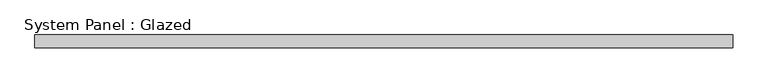
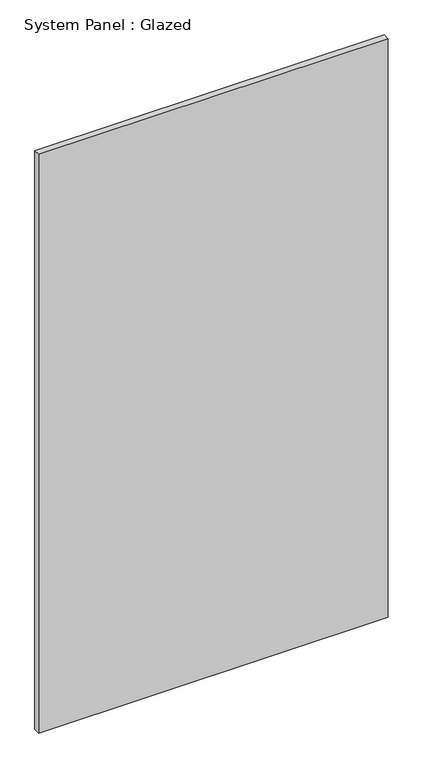
"""IFC4 building model written with IfcOpenShell, lengths in millimetres: plate geometry, System Panel : Glazed."""

from ifc_helpers import new_model, si_unit, origin, origin_with_axes, place, context, project, spatial, polyline, outline, extrude, source, transform, mapped, element, save


def system_panel_glazed_fc6345c6(model_context):
    return source(origin(), model_context, "Body", "SweptSolid", [
        extrude(outline(polyline([(685.8, 24.5), (-685.8, 24.5), (-685.8, 49.5), (685.8, 49.5), (685.8, 24.5)])), origin_with_axes(), (0.0, 0.0, 1.0), 2400.0),
    ])


if __name__ == "__main__":
    model = new_model("IFC4")
    model_context = context("Model", 3, world=origin())
    ifc_project = project(units=[si_unit("LENGTHUNIT", "METRE", prefix="MILLI")], contexts=[model_context])
    site = spatial("IfcSite", under=ifc_project)
    building = spatial("IfcBuilding", under=site)
    placement = place(None, origin())
    system_panel_glazed_shape = system_panel_glazed_fc6345c6(model_context)
    element("IfcPlate", 1, ObjectType="System Panel : Glazed", at=placement, inside=building, context=model_context, shape_type="MappedRepresentation", body=[
        mapped(system_panel_glazed_shape, transform((0.0, 0.0, 0.0), x_axis=(1.0, 0.0, 0.0), y_axis=(0.0, 1.0, 0.0), z_axis=(0.0, 0.0, 1.0))),
    ])
    save(model, "model.ifc")

# Revit data of these elements
# Type "System Panel : Glazed"
#   Keynote = "H11"
#   Construction Type Id = "GSP4R"
#   Analytic Construction = "1/8 in Pilkington single glazing"
#   Visual Light Transmittance = 0.9
#   Solar Heat Gain Coefficient = 0.86
#   Heat Transfer Coefficient (U) = 6.7069 W/(m²·K)
#   Define Thermal Properties by = 1
# Element 1 (IfcPlate, "System Panel : Glazed")
#   Materials on its faces: "Glass"
# Materials
#   "Glass": class "Glass", colour RGB 0 128 192, transparency 0.9, Description = "Soda Lime Glass", Cost = 0
